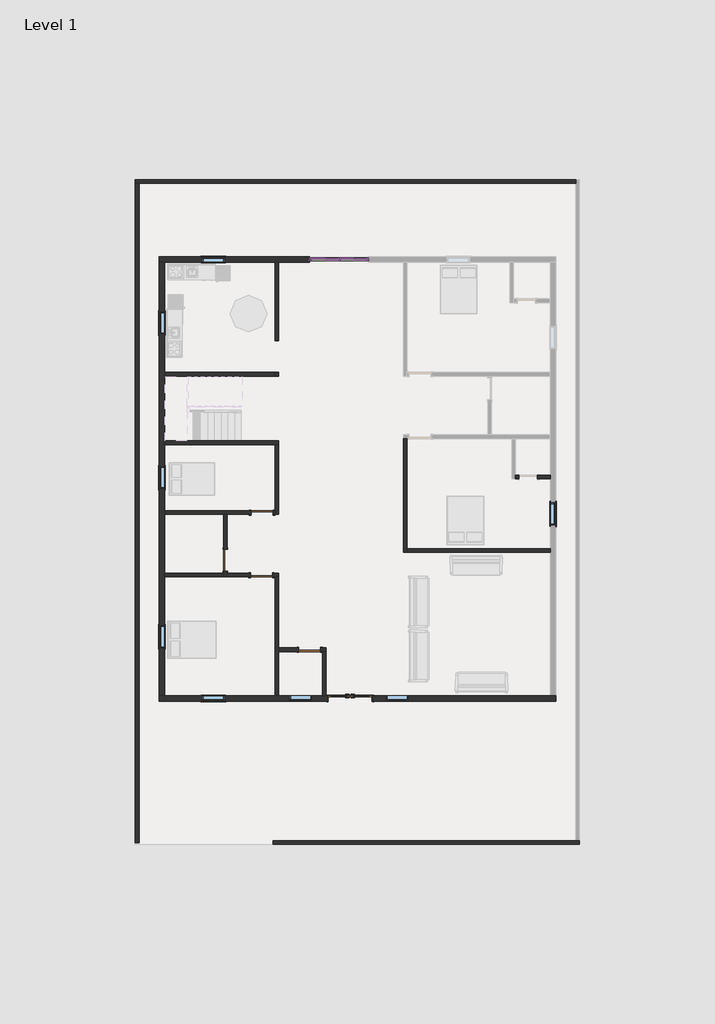
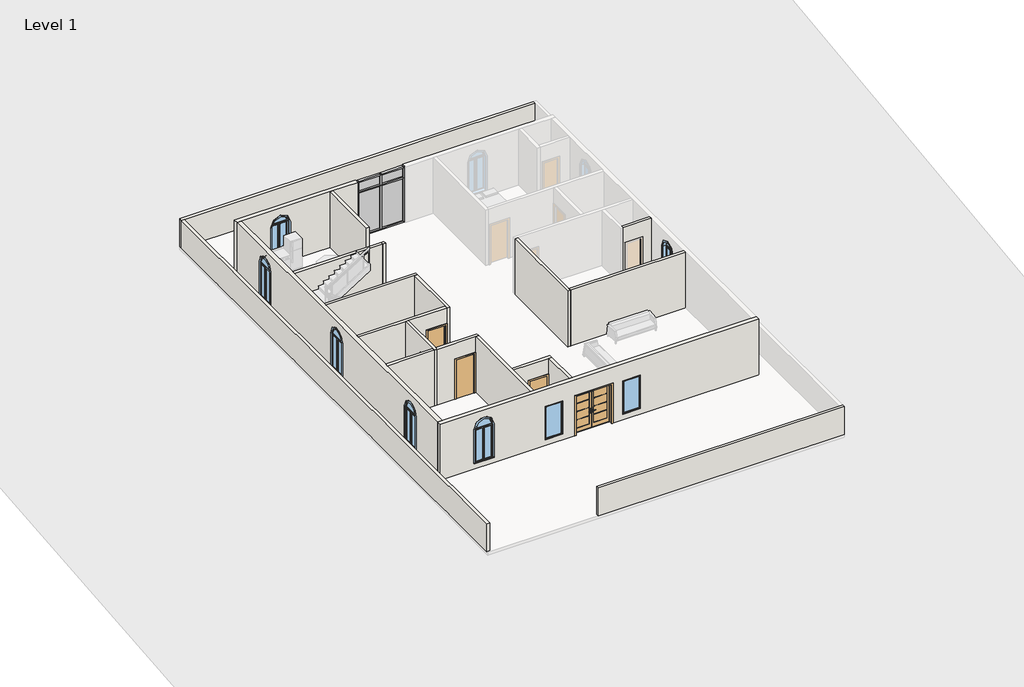
# One storey, part 1 of 2: 21 walls, 12 members, 8 windows, 5 doors, 4 plates.
"""IFC4 building model written with IfcOpenShell, lengths in millimetres."""

from ifc_helpers import new_model, si_unit, frame, origin, origin_with_axes, place, context, project, spatial, polyline, circle_curve, outline, extrude, faceted_brep, transform, mapped, element, save
from ifc_brep_helpers import plane_surface, revolved_surface, advanced_brep
from components import door_5bfea099, door_686f89d2, door_16372e1c, member_e6b9f524, member_866a01fa, member_f0fea5a5, member_6e77e263, member_ee409385, member_47bfaf8a, system_panel_glazed_2148303e, system_panel_glazed_80d043f3, window_e7489165, window_c796fc87

model = new_model("IFC4")

# Units and contexts
model_context = context("Model", 3, world=origin())
ifc_project = project(units=[si_unit("LENGTHUNIT", "METRE", prefix="MILLI")], contexts=[model_context])

# Site, building, storey
site = spatial("IfcSite", under=ifc_project)
building = spatial("IfcBuilding", under=site)
storey = spatial("IfcBuildingStorey", under=building, Name="Level 1", Elevation=0.0)

# Doors
placement = place(None, origin())
door_shape = door_5bfea099(model_context)
element("IfcDoor", 1, ObjectType="Door-Exterior-Double-Full Glass-Wood_Clad : 72\" x 84\"", at=placement, inside=storey, context=model_context, shape_type="MappedRepresentation", body=[
    mapped(door_shape, transform((-1367.6791271, -5663.3296952, 0.0), x_axis=(1.0, 0.0, 0.0), y_axis=(0.0, 1.0, 0.0), z_axis=(0.0, 0.0, 1.0))),
])
door_2_shape = door_686f89d2(model_context)
element("IfcDoor", 2, ObjectType="Single-Flush : 36\" x 84\"", at=placement, inside=storey, context=model_context, shape_type="MappedRepresentation", body=[
    mapped(door_2_shape, transform((-5050.6791271, -548.4046952, 0.0), x_axis=(1.0, 0.0, 0.0), y_axis=(0.0, 1.0, 0.0), z_axis=(0.0, 0.0, 1.0))),
])
element("IfcDoor", 3, ObjectType="Single-Flush : 36\" x 84\"", at=placement, inside=storey, context=model_context, shape_type="MappedRepresentation", body=[
    mapped(door_2_shape, transform((-6549.2791271, 61.1953048, 0.0), x_axis=(0.0, -1.0, 0.0), y_axis=(1.0, 0.0, 0.0), z_axis=(0.0, 0.0, 1.0))),
])
element("IfcDoor", 4, ObjectType="Single-Flush : 36\" x 84\"", at=placement, inside=storey, context=model_context, shape_type="MappedRepresentation", body=[
    mapped(door_2_shape, transform((-3044.0791271, -3647.2046952, 0.0), x_axis=(1.0, 0.0, 0.0), y_axis=(0.0, 1.0, 0.0), z_axis=(0.0, 0.0, 1.0))),
])
door_3_shape = door_16372e1c(model_context)
element("IfcDoor", 5, ObjectType="Single-Flush : 36\" x 84\"", at=placement, inside=storey, context=model_context, shape_type="MappedRepresentation", body=[
    mapped(door_3_shape, transform((-5025.2791271, 2042.3953048, 0.0), x_axis=(1.0, 0.0, 0.0), y_axis=(0.0, 1.0, 0.0), z_axis=(0.0, 0.0, 1.0))),
])

# Members
member_shape = member_e6b9f524(model_context)
element("IfcMember", 6, ObjectType="Rectangular Mullion : 2.5\" x 5\" rectangular", at=placement, inside=storey, context=model_context, shape_type="MappedRepresentation", body=[
    mapped(member_shape, transform((-669.1791271, 12545.2953048, 3048.0), x_axis=(0.0, 0.0, 1.0), y_axis=(0.0, -1.0, 0.0), z_axis=(1.0, 0.0, 0.0))),
])
element("IfcMember", 7, ObjectType="Rectangular Mullion : 2.5\" x 5\" rectangular", at=placement, inside=storey, context=model_context, shape_type="MappedRepresentation", body=[
    mapped(member_shape, transform((-1856.6291271, 12545.2953048, 3048.0), x_axis=(0.0, 0.0, 1.0), y_axis=(0.0, -1.0, 0.0), z_axis=(1.0, 0.0, 0.0))),
])
element("IfcMember", 8, ObjectType="Rectangular Mullion : 2.5\" x 5\" rectangular", at=placement, inside=storey, context=model_context, shape_type="MappedRepresentation", body=[
    mapped(member_shape, transform((-2980.5791271, 12545.2953048, 0.0), x_axis=(0.0, 0.0, -1.0), y_axis=(0.0, -1.0, 0.0), z_axis=(-1.0, 0.0, 0.0))),
])
element("IfcMember", 9, ObjectType="Rectangular Mullion : 2.5\" x 5\" rectangular", at=placement, inside=storey, context=model_context, shape_type="MappedRepresentation", body=[
    mapped(member_shape, transform((-1793.1291271, 12545.2953048, 0.0), x_axis=(0.0, 0.0, -1.0), y_axis=(0.0, -1.0, 0.0), z_axis=(-1.0, 0.0, 0.0))),
])
member_2_shape = member_866a01fa(model_context)
element("IfcMember", 10, ObjectType="Rectangular Mullion : 2.5\" x 5\" rectangular", at=placement, inside=storey, context=model_context, shape_type="MappedRepresentation", body=[
    mapped(member_2_shape, transform((-1856.6291271, 12545.2953048, 2438.4), x_axis=(0.0, 0.0, 1.0), y_axis=(0.0, -1.0, 0.0), z_axis=(1.0, 0.0, 0.0))),
])
element("IfcMember", 11, ObjectType="Rectangular Mullion : 2.5\" x 5\" rectangular", at=placement, inside=storey, context=model_context, shape_type="MappedRepresentation", body=[
    mapped(member_2_shape, transform((-669.1791271, 12545.2953048, 2438.4), x_axis=(0.0, 0.0, 1.0), y_axis=(0.0, -1.0, 0.0), z_axis=(1.0, 0.0, 0.0))),
])
member_3_shape = member_f0fea5a5(model_context)
element("IfcMember", 12, ObjectType="Rectangular Mullion : 2.5\" x 5\" rectangular", at=placement, inside=storey, context=model_context, shape_type="MappedRepresentation", body=[
    mapped(member_3_shape, transform((-1824.8791271, 12545.2953048, 0.0), x_axis=(1.0, 0.0, 0.0), y_axis=(0.0, -1.0, 0.0), z_axis=(0.0, 0.0, -1.0))),
])
member_4_shape = member_6e77e263(model_context)
element("IfcMember", 13, ObjectType="Rectangular Mullion : 2.5\" x 5\" rectangular", at=placement, inside=storey, context=model_context, shape_type="MappedRepresentation", body=[
    mapped(member_4_shape, transform((-1824.8791271, 12545.2953048, 2438.4), x_axis=(1.0, 0.0, 0.0), y_axis=(0.0, -1.0, 0.0), z_axis=(0.0, 0.0, -1.0))),
])
member_5_shape = member_ee409385(model_context)
element("IfcMember", 14, ObjectType="Rectangular Mullion : 2.5\" x 5\" rectangular", at=placement, inside=storey, context=model_context, shape_type="MappedRepresentation", body=[
    mapped(member_5_shape, transform((-605.6791271, 12545.2953048, 0.0), x_axis=(1.0, 0.0, 0.0), y_axis=(0.0, -1.0, 0.0), z_axis=(0.0, 0.0, -1.0))),
])
member_6_shape = member_47bfaf8a(model_context)
element("IfcMember", 15, ObjectType="Rectangular Mullion : 2.5\" x 5\" rectangular", at=placement, inside=storey, context=model_context, shape_type="MappedRepresentation", body=[
    mapped(member_6_shape, transform((-3044.0791271, 12545.2953048, 3048.0), x_axis=(-1.0, 0.0, 0.0), y_axis=(0.0, -1.0, 0.0), z_axis=(0.0, 0.0, 1.0))),
])
element("IfcMember", 16, ObjectType="Rectangular Mullion : 2.5\" x 5\" rectangular", at=placement, inside=storey, context=model_context, shape_type="MappedRepresentation", body=[
    mapped(member_6_shape, transform((-605.6791271, 12545.2953048, 2438.4), x_axis=(1.0, 0.0, 0.0), y_axis=(0.0, -1.0, 0.0), z_axis=(0.0, 0.0, -1.0))),
])
element("IfcMember", 17, ObjectType="Rectangular Mullion : 2.5\" x 5\" rectangular", at=placement, inside=storey, context=model_context, shape_type="MappedRepresentation", body=[
    mapped(member_5_shape, transform((-3044.0791271, 12545.2953048, 2438.4), x_axis=(-1.0, 0.0, 0.0), y_axis=(0.0, -1.0, 0.0), z_axis=(0.0, 0.0, 1.0))),
])

# Plates
system_panel_glazed_shape = system_panel_glazed_2148303e(model_context)
element("IfcPlate", 18, ObjectType="System Panel : Glazed", at=placement, inside=storey, context=model_context, shape_type="MappedRepresentation", body=[
    mapped(system_panel_glazed_shape, transform((-2418.6041271, 12545.2953048, 63.5), x_axis=(1.0, 0.0, 0.0), y_axis=(0.0, 1.0, 0.0), z_axis=(0.0, 0.0, 1.0))),
])
element("IfcPlate", 19, ObjectType="System Panel : Glazed", at=placement, inside=storey, context=model_context, shape_type="MappedRepresentation", body=[
    mapped(system_panel_glazed_shape, transform((-1231.1541271, 12545.2953048, 63.5), x_axis=(1.0, 0.0, 0.0), y_axis=(0.0, 1.0, 0.0), z_axis=(0.0, 0.0, 1.0))),
])
system_panel_glazed_2_shape = system_panel_glazed_80d043f3(model_context)
element("IfcPlate", 20, ObjectType="System Panel : Glazed", at=placement, inside=storey, context=model_context, shape_type="MappedRepresentation", body=[
    mapped(system_panel_glazed_2_shape, transform((-2418.6041271, 12545.2953048, 2470.15), x_axis=(1.0, 0.0, 0.0), y_axis=(0.0, 1.0, 0.0), z_axis=(0.0, 0.0, 1.0))),
])
element("IfcPlate", 21, ObjectType="System Panel : Glazed", at=placement, inside=storey, context=model_context, shape_type="MappedRepresentation", body=[
    mapped(system_panel_glazed_2_shape, transform((-1231.1541271, 12545.2953048, 2470.15), x_axis=(1.0, 0.0, 0.0), y_axis=(0.0, 1.0, 0.0), z_axis=(0.0, 0.0, 1.0))),
])

# Walls
element("IfcWall", 22, ObjectType="6\"", at=placement, inside=storey, context=model_context, shape_type="Brep", body=[
    faceted_brep([(-10283.0791271, 15707.5953048, 0.0), (-10130.6791271, 15707.5953048, 0.0), (8004.9208729, 15707.5953048, 0.0), (8004.9208729, 15707.5953048, 1524.0), (-10130.6791271, 15707.5953048, 1524.0), (-10283.0791271, 15707.5953048, 1524.0), (-10283.0791271, 15859.9953048, 0.0), (-10283.0791271, 15859.9953048, 1524.0), (8004.9208729, 15859.9953048, 1524.0), (8004.9208729, 15859.9953048, 0.0)], [[[0, 1, 2, 3, 4, 5]], [[6, 7, 8, 9]], [[2, 1, 0, 6, 9]], [[5, 4, 3, 8, 7]], [[0, 5, 7, 6]], [[3, 2, 9, 8]]]),
])
element("IfcWall", 23, ObjectType="6\"", at=placement, inside=storey, context=model_context, shape_type="SweptSolid", body=[
    extrude(outline(polyline([(-10130.6791271, 15707.5953048), (-10130.6791271, -11648.2046952), (-10283.0791271, -11648.2046952), (-10283.0791271, 15707.5953048), (-10130.6791271, 15707.5953048)])), origin_with_axes(), (0.0, 0.0, 1.0), 1524.0),
])
element("IfcWall", 24, ObjectType="6\"", at=placement, inside=storey, context=model_context, shape_type="Brep", body=[
    faceted_brep([(8157.3208729, -11572.0046952, 0.0), (8004.9208729, -11572.0046952, 0.0), (-4568.0791271, -11572.0046952, 0.0), (-4568.0791271, -11572.0046952, 1524.0), (8004.9208729, -11572.0046952, 1524.0), (8157.3208729, -11572.0046952, 1524.0), (8157.3208729, -11724.4046952, 0.0), (8157.3208729, -11724.4046952, 1524.0), (-4568.0791271, -11724.4046952, 1524.0), (-4568.0791271, -11724.4046952, 0.0)], [[[0, 1, 2, 3, 4, 5]], [[6, 7, 8, 9]], [[2, 1, 0, 6, 9]], [[3, 2, 9, 8]], [[5, 4, 3, 8, 7]], [[0, 5, 7, 6]]]),
])
element("IfcWall", 25, ObjectType="6\"", at=placement, inside=storey, context=model_context, shape_type="SweptSolid", body=[
    extrude(outline(polyline([(-4491.8791271, 9167.0953048), (-4491.8791271, 12430.9953048), (-4339.4791271, 12430.9953048), (-4339.4791271, 9167.0953048), (-4491.8791271, 9167.0953048)])), origin_with_axes(), (0.0, 0.0, 1.0), 3048.0),
])
element("IfcWall", 26, ObjectType="6\"", at=placement, inside=storey, context=model_context, shape_type="SweptSolid", body=[
    extrude(outline(polyline([(-9063.8791271, 7858.9953048), (-4491.8791271, 7858.9953048), (-4491.8791271, 7706.5953048), (-9063.8791271, 7706.5953048), (-9063.8791271, 7858.9953048)])), origin_with_axes(), (0.0, 0.0, 1.0), 3048.0),
])
element("IfcWall", 27, ObjectType="6\"", at=placement, inside=storey, context=model_context, shape_type="Brep", body=[
    faceted_brep([(842.1208729, 5115.7953048, 0.0), (842.1208729, 391.3953048, 0.0), (842.1208729, 391.3953048, 3048.0), (842.1208729, 5115.7953048, 3048.0), (994.5208729, 5115.7953048, 0.0), (994.5208729, 5115.7953048, 3048.0), (994.5208729, 543.7953048, 3048.0), (994.5208729, 391.3953048, 3048.0), (994.5208729, 391.3953048, 0.0), (994.5208729, 543.7953048, 0.0)], [[[0, 1, 2, 3]], [[4, 5, 6, 7, 8, 9]], [[1, 0, 4, 9, 8]], [[3, 2, 7, 6, 5]], [[2, 1, 8, 7]], [[0, 3, 5, 4]]]),
])
element("IfcWall", 28, ObjectType="6\"", at=placement, inside=storey, context=model_context, shape_type="SweptSolid", body=[
    extrude(outline(polyline([(6938.1208729, 391.3953048), (994.5208729, 391.3953048), (994.5208729, 543.7953048), (6938.1208729, 543.7953048), (6938.1208729, 391.3953048)])), origin_with_axes(), (0.0, 0.0, 1.0), 3048.0),
])
element("IfcWall", 29, ObjectType="6\"", at=placement, inside=storey, context=model_context, shape_type="Brep", body=[
    faceted_brep([(-9063.8791271, 4861.7953048, 0.0), (-4491.8791271, 4861.7953048, 0.0), (-4339.4791271, 4861.7953048, 0.0), (-4339.4791271, 4861.7953048, 3048.0), (-4491.8791271, 4861.7953048, 3048.0), (-9063.8791271, 4861.7953048, 3048.0), (-9063.8791271, 5014.1953048, 0.0), (-9063.8791271, 5014.1953048, 3048.0), (-4339.4791271, 5014.1953048, 3048.0), (-4339.4791271, 5014.1953048, 0.0)], [[[0, 1, 2, 3, 4, 5]], [[6, 7, 8, 9]], [[2, 1, 0, 6, 9]], [[5, 4, 3, 8, 7]], [[3, 2, 9, 8]], [[0, 5, 7, 6]]]),
])
element("IfcWall", 30, ObjectType="6\"", at=placement, inside=storey, context=model_context, shape_type="Brep", body=[
    faceted_brep([(-4491.8791271, 4861.7953048, 0.0), (-4491.8791271, 2118.5953048, 0.0), (-4491.8791271, 1966.1953048, 0.0), (-4491.8791271, 1966.1953048, 3048.0), (-4491.8791271, 2118.5953048, 3048.0), (-4491.8791271, 4861.7953048, 3048.0), (-4339.4791271, 4861.7953048, 0.0), (-4339.4791271, 4861.7953048, 3048.0), (-4339.4791271, 1966.1953048, 3048.0), (-4339.4791271, 1966.1953048, 0.0)], [[[0, 1, 2, 3, 4, 5]], [[6, 7, 8, 9]], [[2, 1, 0, 6, 9]], [[5, 4, 3, 8, 7]], [[0, 5, 7, 6]], [[3, 2, 9, 8]]]),
])
element("IfcWall", 31, ObjectType="6\"", at=placement, inside=storey, context=model_context, shape_type="Brep", body=[
    faceted_brep([(-4491.8791271, 2118.5953048, 0.0), (-4568.0791271, 2118.5953048, 0.0), (-4568.0791271, 2118.5953048, 2133.6), (-5482.4791271, 2118.5953048, 2133.6), (-5482.4791271, 2118.5953048, 0.0), (-9063.8791271, 2118.5953048, 0.0), (-9063.8791271, 2118.5953048, 3048.0), (-4491.8791271, 2118.5953048, 3048.0), (-4568.0791271, 1966.1953048, 2133.6), (-4568.0791271, 1966.1953048, 0.0), (-4491.8791271, 1966.1953048, 0.0), (-4491.8791271, 1966.1953048, 3048.0), (-6473.0791271, 1966.1953048, 3048.0), (-6625.4791271, 1966.1953048, 3048.0), (-9063.8791271, 1966.1953048, 3048.0), (-9063.8791271, 1966.1953048, 0.0), (-6625.4791271, 1966.1953048, 0.0), (-6473.0791271, 1966.1953048, 0.0), (-5482.4791271, 1966.1953048, 0.0), (-5482.4791271, 1966.1953048, 2133.6)], [[[0, 1, 2, 3, 4, 5, 6, 7]], [[8, 9, 10, 11, 12, 13, 14, 15, 16, 17, 18, 19]], [[10, 9, 1, 0]], [[18, 17, 16, 15, 5, 4]], [[7, 6, 14, 13, 12, 11]], [[0, 7, 11, 10]], [[6, 5, 15, 14]], [[2, 1, 9, 8]], [[3, 2, 8, 19]], [[4, 3, 19, 18]]]),
])
element("IfcWall", 32, ObjectType="6\"", at=placement, inside=storey, context=model_context, shape_type="Brep", body=[
    faceted_brep([(-6625.4791271, -396.0046952, 2133.6), (-6625.4791271, -396.0046952, 0.0), (-6625.4791271, -472.2046952, 0.0), (-6625.4791271, -624.6046952, 0.0), (-6625.4791271, -624.6046952, 3048.0), (-6625.4791271, -472.2046952, 3048.0), (-6625.4791271, 1966.1953048, 3048.0), (-6625.4791271, 1966.1953048, 0.0), (-6625.4791271, 518.3953048, 0.0), (-6625.4791271, 518.3953048, 2133.6), (-6473.0791271, -624.6046952, 0.0), (-6473.0791271, -472.2046952, 0.0), (-6473.0791271, -396.0046952, 0.0), (-6473.0791271, -396.0046952, 2133.6), (-6473.0791271, 518.3953048, 2133.6), (-6473.0791271, 518.3953048, 0.0), (-6473.0791271, 1966.1953048, 0.0), (-6473.0791271, 1966.1953048, 3048.0), (-6473.0791271, -472.2046952, 3048.0), (-6473.0791271, -624.6046952, 3048.0)], [[[0, 1, 2, 3, 4, 5, 6, 7, 8, 9]], [[10, 11, 12, 13, 14, 15, 16, 17, 18, 19]], [[8, 7, 16, 15]], [[3, 2, 1, 12, 11, 10]], [[6, 5, 4, 19, 18, 17]], [[7, 6, 17, 16]], [[4, 3, 10, 19]], [[13, 12, 1, 0]], [[14, 13, 0, 9]], [[15, 14, 9, 8]]]),
])
element("IfcWall", 33, ObjectType="6\"", at=placement, inside=storey, context=model_context, shape_type="SweptSolid", body=[
    extrude(outline(polyline([(-9063.8791271, -472.2046952), (-6625.4791271, -472.2046952), (-6625.4791271, -624.6046952), (-9063.8791271, -624.6046952), (-9063.8791271, -472.2046952)])), origin_with_axes(), (0.0, 0.0, 1.0), 3048.0),
])
element("IfcWall", 34, ObjectType="6\"", at=placement, inside=storey, context=model_context, shape_type="Brep", body=[
    faceted_brep([(-4593.4791271, -624.6046952, 2133.6), (-4593.4791271, -624.6046952, 0.0), (-4491.8791271, -624.6046952, 0.0), (-4339.4791271, -624.6046952, 0.0), (-4339.4791271, -624.6046952, 3048.0), (-4491.8791271, -624.6046952, 3048.0), (-6473.0791271, -624.6046952, 3048.0), (-6473.0791271, -624.6046952, 0.0), (-5507.8791271, -624.6046952, 0.0), (-5507.8791271, -624.6046952, 2133.6), (-4339.4791271, -472.2046952, 0.0), (-4593.4791271, -472.2046952, 0.0), (-4593.4791271, -472.2046952, 2133.6), (-5507.8791271, -472.2046952, 2133.6), (-5507.8791271, -472.2046952, 0.0), (-6473.0791271, -472.2046952, 0.0), (-6473.0791271, -472.2046952, 3048.0), (-4339.4791271, -472.2046952, 3048.0)], [[[0, 1, 2, 3, 4, 5, 6, 7, 8, 9]], [[10, 11, 12, 13, 14, 15, 16, 17]], [[8, 7, 15, 14]], [[3, 2, 1, 11, 10]], [[6, 5, 4, 17, 16]], [[7, 6, 16, 15]], [[4, 3, 10, 17]], [[12, 11, 1, 0]], [[13, 12, 0, 9]], [[14, 13, 9, 8]]]),
])
element("IfcWall", 35, ObjectType="6\"", at=placement, inside=storey, context=model_context, shape_type="Brep", body=[
    faceted_brep([(-4491.8791271, -624.6046952, 0.0), (-4491.8791271, -5552.2046952, 0.0), (-4491.8791271, -5552.2046952, 3048.0), (-4491.8791271, -624.6046952, 3048.0), (-4339.4791271, -624.6046952, 0.0), (-4339.4791271, -624.6046952, 3048.0), (-4339.4791271, -3571.0046952, 3048.0), (-4339.4791271, -3723.4046952, 3048.0), (-4339.4791271, -5552.2046952, 3048.0), (-4339.4791271, -5552.2046952, 0.0), (-4339.4791271, -3723.4046952, 0.0), (-4339.4791271, -3571.0046952, 0.0)], [[[0, 1, 2, 3]], [[4, 5, 6, 7, 8, 9, 10, 11]], [[1, 0, 4, 11, 10, 9]], [[3, 2, 8, 7, 6, 5]], [[0, 3, 5, 4]], [[2, 1, 9, 8]]]),
])
element("IfcWall", 36, ObjectType="6\"", at=placement, inside=storey, context=model_context, shape_type="Brep", body=[
    faceted_brep([(-2586.8791271, -3723.4046952, 2133.6), (-2586.8791271, -3723.4046952, 0.0), (-2510.6791271, -3723.4046952, 0.0), (-2358.2791271, -3723.4046952, 0.0), (-2358.2791271, -3723.4046952, 3048.0), (-2510.6791271, -3723.4046952, 3048.0), (-4339.4791271, -3723.4046952, 3048.0), (-4339.4791271, -3723.4046952, 0.0), (-3501.2791271, -3723.4046952, 0.0), (-3501.2791271, -3723.4046952, 2133.6), (-2358.2791271, -3571.0046952, 0.0), (-2586.8791271, -3571.0046952, 0.0), (-2586.8791271, -3571.0046952, 2133.6), (-3501.2791271, -3571.0046952, 2133.6), (-3501.2791271, -3571.0046952, 0.0), (-4339.4791271, -3571.0046952, 0.0), (-4339.4791271, -3571.0046952, 3048.0), (-2358.2791271, -3571.0046952, 3048.0)], [[[0, 1, 2, 3, 4, 5, 6, 7, 8, 9]], [[10, 11, 12, 13, 14, 15, 16, 17]], [[8, 7, 15, 14]], [[3, 2, 1, 11, 10]], [[6, 5, 4, 17, 16]], [[7, 6, 16, 15]], [[4, 3, 10, 17]], [[12, 11, 1, 0]], [[13, 12, 0, 9]], [[14, 13, 9, 8]]]),
])
element("IfcWall", 37, ObjectType="6\"", at=placement, inside=storey, context=model_context, shape_type="SweptSolid", body=[
    extrude(outline(polyline([(-2510.6791271, -5552.2046952), (-2510.6791271, -3723.4046952), (-2358.2791271, -3723.4046952), (-2358.2791271, -5552.2046952), (-2510.6791271, -5552.2046952)])), origin_with_axes(), (0.0, 0.0, 1.0), 3048.0),
])
element("IfcWall", 38, ObjectType="6\"", at=placement, inside=storey, context=model_context, shape_type="SweptSolid", body=[
    extrude(outline(polyline([(0.0, 5490.3208729), (0.0, 5642.7208729), (2133.6, 5642.7208729), (2133.6, 6404.7208729), (0.0, 6404.7208729), (0.0, 6938.1208729), (3048.0, 6938.1208729), (3048.0, 5490.3208729), (0.0, 5490.3208729)])), frame((0.0, 3439.3953048, 0.0), z_axis=(0.0, 1.0, 0.0), x_axis=(0.0, 0.0, 1.0)), (0.0, 0.0, 1.0), 152.4),
])
element("IfcWall", 39, ObjectType="6\"", at=placement, inside=storey, context=model_context, shape_type="SweptSolid", body=[
    extrude(outline(polyline([(-4491.8791271, 7706.5953048), (-4491.8791271, 7858.9953048), (-4339.4791271, 7858.9953048), (-4339.4791271, 7706.5953048), (-4491.8791271, 7706.5953048)])), origin_with_axes(), (0.0, 0.0, 1.0), 3048.0),
])
element("IfcWall", 40, ObjectType="9\"", at=placement, inside=storey, context=model_context, shape_type="AdvancedBrep", body=[
    advanced_brep(
    [(-9292.4791271, 12430.9953048, 0.0), (-9063.8791271, 12430.9953048, 0.0), (-4491.8791271, 12430.9953048, 0.0), (-4339.4791271, 12430.9953048, 0.0), (-3044.0791271, 12430.9953048, 0.0), (-3044.0791271, 12430.9953048, 3048.0), (-4339.4791271, 12430.9953048, 3048.0), (-4491.8791271, 12430.9953048, 3048.0), (-9063.8791271, 12430.9953048, 3048.0), (-9292.4791271, 12430.9953048, 3048.0), (-6587.3791271, 12430.9953048, 2152.65), (-6587.3791271, 12430.9953048, 304.8), (-7501.7791271, 12430.9953048, 304.8), (-7501.7791271, 12430.9953048, 2152.65), (-9292.4791271, 12659.5953048, 0.0), (-9292.4791271, 12659.5953048, 3048.0), (-3044.0791271, 12659.5953048, 3048.0), (-3044.0791271, 12659.5953048, 0.0), (-6587.3791271, 12659.5953048, 2152.65), (-7501.7791271, 12659.5953048, 2152.65), (-7501.7791271, 12659.5953048, 304.8), (-6587.3791271, 12659.5953048, 304.8)],
    [
        (0, 1),
        (1, 2),
        (2, 3),
        (3, 4),
        (4, 5),
        (5, 6),
        (6, 7),
        (7, 8),
        (8, 9),
        (9, 0),
        (10, 11),
        (11, 12),
        (12, 13),
        (13, 10, circle_curve(frame((-7044.5791271, 12430.9953048, 2152.65), z_axis=(0.0, 1.0, 0.0), x_axis=(1.0, 0.0, 0.0)), 457.2)),
        (14, 15),
        (15, 16),
        (16, 17),
        (17, 14),
        (18, 19, circle_curve(frame((-7044.5791271, 12659.5953048, 2152.65), z_axis=(0.0, -1.0, 0.0), x_axis=(1.0, 0.0, 0.0)), 457.2)),
        (19, 20),
        (20, 21),
        (21, 18),
        (0, 14),
        (17, 4),
        (16, 5),
        (15, 9),
        (10, 18),
        (21, 11),
        (20, 12),
        (19, 13),
    ],
    [
        plane_surface(frame((-10130.6791271, 12430.9953048, 0.0), z_axis=(0.0, -1.0, 0.0), x_axis=(1.0, 0.0, 0.0))),
        plane_surface(frame((-10130.6791271, 12659.5953048, 0.0), z_axis=(0.0, 1.0, 0.0), x_axis=(-1.0, 0.0, 0.0))),
        plane_surface(frame((-9292.4791271, 12430.9953048, 0.0), z_axis=(0.0, 0.0, -1.0), x_axis=(0.0, 1.0, 0.0))),
        plane_surface(frame((-3044.0791271, 12430.9953048, 0.0), z_axis=(1.0, 0.0, 0.0), x_axis=(0.0, 1.0, 0.0))),
        plane_surface(frame((-3044.0791271, 12430.9953048, 3048.0), z_axis=(0.0, 0.0, 1.0), x_axis=(0.0, 1.0, 0.0))),
        plane_surface(frame((-9292.4791271, 12430.9953048, 3048.0), z_axis=(-1.0, 0.0, 0.0), x_axis=(0.0, 1.0, 0.0))),
        plane_surface(frame((-6587.3791271, 12430.9953048, 2152.65), z_axis=(-1.0, 0.0, 0.0), x_axis=(0.0, 1.0, 0.0))),
        plane_surface(frame((-6587.3791271, 12430.9953048, 304.8), z_axis=(0.0, 0.0, 1.0), x_axis=(0.0, 1.0, 0.0))),
        plane_surface(frame((-7501.7791271, 12430.9953048, 304.8), z_axis=(1.0, 0.0, 0.0), x_axis=(0.0, 1.0, 0.0))),
        revolved_surface(polyline([(-6587.3791271, 12659.5953048, 2152.65), (-6587.3791271, 12430.9953048, 2152.65)]), (-7044.5791271, 12430.9953048, 2152.65), (0.0, 1.0, 0.0)),
    ],
    [
        (0, [[1, 2, 3, 4, 5, 6, 7, 8, 9, 10], [11, 12, 13, 14]]),
        (1, [[15, 16, 17, 18], [19, 20, 21, 22]]),
        (2, [[-4, -3, -2, -1, 23, -18, 24]]),
        (3, [[-5, -24, -17, 25]]),
        (4, [[-9, -8, -7, -6, -25, -16, 26]]),
        (5, [[-10, -26, -15, -23]]),
        (6, [[-11, 27, -22, 28]]),
        (7, [[-12, -28, -21, 29]]),
        (8, [[-13, -29, -20, 30]]),
        (9, [[-14, -30, -19, -27]]),
    ],
),
])
element("IfcWall", 41, ObjectType="9\"", at=placement, inside=storey, context=model_context, shape_type="AdvancedBrep", body=[
    advanced_brep(
    [(-9292.4791271, 12430.9953048, 0.0), (-9292.4791271, -5552.2046952, 0.0), (-9292.4791271, -5552.2046952, 3048.0), (-9292.4791271, 12430.9953048, 3048.0), (-9292.4791271, -2650.2546952, 2152.65), (-9292.4791271, -3564.6546952, 2152.65), (-9292.4791271, -3564.6546952, 304.8), (-9292.4791271, -2650.2546952, 304.8), (-9292.4791271, 3947.3953048, 2152.65), (-9292.4791271, 3032.9953048, 2152.65), (-9292.4791271, 3032.9953048, 304.8), (-9292.4791271, 3947.3953048, 304.8), (-9292.4791271, 10367.2453048, 2152.65), (-9292.4791271, 9452.8453048, 2152.65), (-9292.4791271, 9452.8453048, 304.8), (-9292.4791271, 10367.2453048, 304.8), (-9063.8791271, 12430.9953048, 0.0), (-9063.8791271, 12430.9953048, 3048.0), (-9063.8791271, 7858.9953048, 3048.0), (-9063.8791271, 7706.5953048, 3048.0), (-9063.8791271, 5014.1953048, 3048.0), (-9063.8791271, 4861.7953048, 3048.0), (-9063.8791271, 2118.5953048, 3048.0), (-9063.8791271, 1966.1953048, 3048.0), (-9063.8791271, -472.2046952, 3048.0), (-9063.8791271, -624.6046952, 3048.0), (-9063.8791271, -5552.2046952, 3048.0), (-9063.8791271, -5552.2046952, 0.0), (-9063.8791271, -624.6046952, 0.0), (-9063.8791271, -472.2046952, 0.0), (-9063.8791271, 1966.1953048, 0.0), (-9063.8791271, 2118.5953048, 0.0), (-9063.8791271, 4861.7953048, 0.0), (-9063.8791271, 5014.1953048, 0.0), (-9063.8791271, 7706.5953048, 0.0), (-9063.8791271, 7858.9953048, 0.0), (-9063.8791271, -2650.2546952, 2152.65), (-9063.8791271, -2650.2546952, 304.8), (-9063.8791271, -3564.6546952, 304.8), (-9063.8791271, -3564.6546952, 2152.65), (-9063.8791271, 3947.3953048, 2152.65), (-9063.8791271, 3947.3953048, 304.8), (-9063.8791271, 3032.9953048, 304.8), (-9063.8791271, 3032.9953048, 2152.65), (-9063.8791271, 10367.2453048, 2152.65), (-9063.8791271, 10367.2453048, 304.8), (-9063.8791271, 9452.8453048, 304.8), (-9063.8791271, 9452.8453048, 2152.65)],
    [
        (0, 1),
        (1, 2),
        (2, 3),
        (3, 0),
        (4, 5, circle_curve(frame((-9292.4791271, -3107.4546952, 2152.65), z_axis=(1.0, 0.0, 0.0), x_axis=(0.0, 1.0, 0.0)), 457.2)),
        (5, 6),
        (6, 7),
        (7, 4),
        (8, 9, circle_curve(frame((-9292.4791271, 3490.1953048, 2152.65), z_axis=(1.0, 0.0, 0.0), x_axis=(0.0, 1.0, 0.0)), 457.2)),
        (9, 10),
        (10, 11),
        (11, 8),
        (12, 13, circle_curve(frame((-9292.4791271, 9910.0453048, 2152.65), z_axis=(1.0, 0.0, 0.0), x_axis=(0.0, 1.0, 0.0)), 457.2)),
        (13, 14),
        (14, 15),
        (15, 12),
        (16, 17),
        (17, 18),
        (18, 19),
        (19, 20),
        (20, 21),
        (21, 22),
        (22, 23),
        (23, 24),
        (24, 25),
        (25, 26),
        (26, 27),
        (27, 28),
        (28, 29),
        (29, 30),
        (30, 31),
        (31, 32),
        (32, 33),
        (33, 34),
        (34, 35),
        (35, 16),
        (36, 37),
        (37, 38),
        (38, 39),
        (39, 36, circle_curve(frame((-9063.8791271, -3107.4546952, 2152.65), z_axis=(-1.0, 0.0, 0.0), x_axis=(0.0, 1.0, 0.0)), 457.2)),
        (40, 41),
        (41, 42),
        (42, 43),
        (43, 40, circle_curve(frame((-9063.8791271, 3490.1953048, 2152.65), z_axis=(-1.0, 0.0, 0.0), x_axis=(0.0, 1.0, 0.0)), 457.2)),
        (44, 45),
        (45, 46),
        (46, 47),
        (47, 44, circle_curve(frame((-9063.8791271, 9910.0453048, 2152.65), z_axis=(-1.0, 0.0, 0.0), x_axis=(0.0, 1.0, 0.0)), 457.2)),
        (0, 16),
        (27, 1),
        (2, 26),
        (17, 3),
        (36, 4),
        (7, 37),
        (6, 38),
        (5, 39),
        (40, 8),
        (11, 41),
        (10, 42),
        (9, 43),
        (44, 12),
        (15, 45),
        (14, 46),
        (13, 47),
    ],
    [
        plane_surface(frame((-9292.4791271, 12430.9953048, 0.0), z_axis=(-1.0, 0.0, 0.0), x_axis=(0.0, -1.0, 0.0))),
        plane_surface(frame((-9063.8791271, 12430.9953048, 0.0), z_axis=(1.0, 0.0, 0.0), x_axis=(0.0, 1.0, 0.0))),
        plane_surface(frame((-9292.4791271, 12545.2953048, 0.0), z_axis=(0.0, 0.0, -1.0), x_axis=(1.0, 0.0, 0.0))),
        plane_surface(frame((-9292.4791271, -5666.5046952, 3048.0), z_axis=(0.0, 0.0, 1.0), x_axis=(1.0, 0.0, 0.0))),
        plane_surface(frame((-10130.6791271, 12430.9953048, 0.0), z_axis=(0.0, 1.0, 0.0), x_axis=(1.0, 0.0, 0.0))),
        plane_surface(frame((-10130.6791271, -5552.2046952, 0.0), z_axis=(0.0, -1.0, 0.0), x_axis=(-1.0, 0.0, 0.0))),
        plane_surface(frame((-9063.8791271, -2650.2546952, 2152.65), z_axis=(0.0, -1.0, 0.0), x_axis=(-1.0, 0.0, 0.0))),
        plane_surface(frame((-9063.8791271, -2650.2546952, 304.8), z_axis=(0.0, 0.0, 1.0), x_axis=(-1.0, 0.0, 0.0))),
        plane_surface(frame((-9063.8791271, -3564.6546952, 304.8), z_axis=(0.0, 1.0, 0.0), x_axis=(-1.0, 0.0, 0.0))),
        revolved_surface(polyline([(-9292.4791271, -2650.2546952000002, 2152.65), (-9063.8791271, -2650.2546952000002, 2152.65)]), (-9063.8791271, -3107.4546952, 2152.65), (-1.0, 0.0, 0.0)),
        plane_surface(frame((-9063.8791271, 3947.3953048, 2152.65), z_axis=(0.0, -1.0, 0.0), x_axis=(-1.0, 0.0, 0.0))),
        plane_surface(frame((-9063.8791271, 3947.3953048, 304.8), z_axis=(0.0, 0.0, 1.0), x_axis=(-1.0, 0.0, 0.0))),
        plane_surface(frame((-9063.8791271, 3032.9953048, 304.8), z_axis=(0.0, 1.0, 0.0), x_axis=(-1.0, 0.0, 0.0))),
        revolved_surface(polyline([(-9292.4791271, 3947.3953048, 2152.65), (-9063.8791271, 3947.3953048, 2152.65)]), (-9063.8791271, 3490.1953048, 2152.65), (-1.0, 0.0, 0.0)),
        plane_surface(frame((-9063.8791271, 10367.2453048, 2152.65), z_axis=(0.0, -1.0, 0.0), x_axis=(-1.0, 0.0, 0.0))),
        plane_surface(frame((-9063.8791271, 10367.2453048, 304.8), z_axis=(0.0, 0.0, 1.0), x_axis=(-1.0, 0.0, 0.0))),
        plane_surface(frame((-9063.8791271, 9452.8453048, 304.8), z_axis=(0.0, 1.0, 0.0), x_axis=(-1.0, 0.0, 0.0))),
        revolved_surface(polyline([(-9292.4791271, 10367.2453048, 2152.65), (-9063.8791271, 10367.2453048, 2152.65)]), (-9063.8791271, 9910.0453048, 2152.65), (-1.0, 0.0, 0.0)),
    ],
    [
        (0, [[1, 2, 3, 4], [5, 6, 7, 8], [9, 10, 11, 12], [13, 14, 15, 16]]),
        (1, [[17, 18, 19, 20, 21, 22, 23, 24, 25, 26, 27, 28, 29, 30, 31, 32, 33, 34, 35, 36], [37, 38, 39, 40], [41, 42, 43, 44], [45, 46, 47, 48]]),
        (2, [[-1, 49, -36, -35, -34, -33, -32, -31, -30, -29, -28, 50]]),
        (3, [[-3, 51, -26, -25, -24, -23, -22, -21, -20, -19, -18, 52]]),
        (4, [[-4, -52, -17, -49]]),
        (5, [[-2, -50, -27, -51]]),
        (6, [[-37, 53, -8, 54]]),
        (7, [[-38, -54, -7, 55]]),
        (8, [[-39, -55, -6, 56]]),
        (9, [[-40, -56, -5, -53]]),
        (10, [[-41, 57, -12, 58]]),
        (11, [[-42, -58, -11, 59]]),
        (12, [[-43, -59, -10, 60]]),
        (13, [[-44, -60, -9, -57]]),
        (14, [[-45, 61, -16, 62]]),
        (15, [[-46, -62, -15, 63]]),
        (16, [[-47, -63, -14, 64]]),
        (17, [[-48, -64, -13, -61]]),
    ],
),
])
element("IfcWall", 42, ObjectType="9\"", at=placement, inside=storey, context=model_context, shape_type="AdvancedBrep", body=[
    advanced_brep(
    [(7166.7208729, -5780.8046952, 0.0), (7166.7208729, -5780.8046952, 3048.0), (-9292.4791271, -5780.8046952, 3048.0), (-9292.4791271, -5780.8046952, 0.0), (-2307.4791271, -5780.8046952, 0.0), (-2307.4791271, -5780.8046952, 2159.0), (-427.8791271, -5780.8046952, 2159.0), (-427.8791271, -5780.8046952, 0.0), (-7501.7791271, -5780.8046952, 2152.65), (-6587.3791271, -5780.8046952, 2152.65), (-6587.3791271, -5780.8046952, 304.8), (-7501.7791271, -5780.8046952, 304.8), (130.9208729, -5780.8046952, 2133.6), (1045.3208729, -5780.8046952, 2133.6), (1045.3208729, -5780.8046952, 304.8), (130.9208729, -5780.8046952, 304.8), (-3882.2791271, -5780.8046952, 2133.6), (-2967.8791271, -5780.8046952, 2133.6), (-2967.8791271, -5780.8046952, 304.8), (-3882.2791271, -5780.8046952, 304.8), (7166.7208729, -5552.2046952, 3048.0), (7166.7208729, -5552.2046952, 0.0), (6938.1208729, -5552.2046952, 0.0), (-427.8791271, -5552.2046952, 0.0), (-427.8791271, -5552.2046952, 2159.0), (-2307.4791271, -5552.2046952, 2159.0), (-2307.4791271, -5552.2046952, 0.0), (-2358.2791271, -5552.2046952, 0.0), (-2510.6791271, -5552.2046952, 0.0), (-4339.4791271, -5552.2046952, 0.0), (-4491.8791271, -5552.2046952, 0.0), (-9063.8791271, -5552.2046952, 0.0), (-9292.4791271, -5552.2046952, 0.0), (-9292.4791271, -5552.2046952, 3048.0), (-9063.8791271, -5552.2046952, 3048.0), (-4491.8791271, -5552.2046952, 3048.0), (-4339.4791271, -5552.2046952, 3048.0), (-2510.6791271, -5552.2046952, 3048.0), (-2358.2791271, -5552.2046952, 3048.0), (6938.1208729, -5552.2046952, 3048.0), (-7501.7791271, -5552.2046952, 2152.65), (-7501.7791271, -5552.2046952, 304.8), (-6587.3791271, -5552.2046952, 304.8), (-6587.3791271, -5552.2046952, 2152.65), (130.9208729, -5552.2046952, 2133.6), (130.9208729, -5552.2046952, 304.8), (1045.3208729, -5552.2046952, 304.8), (1045.3208729, -5552.2046952, 2133.6), (-3882.2791271, -5552.2046952, 2133.6), (-3882.2791271, -5552.2046952, 304.8), (-2967.8791271, -5552.2046952, 304.8), (-2967.8791271, -5552.2046952, 2133.6)],
    [
        (0, 1),
        (1, 2),
        (2, 3),
        (3, 4),
        (4, 5),
        (5, 6),
        (6, 7),
        (7, 0),
        (8, 9, circle_curve(frame((-7044.5791271, -5780.8046952, 2152.65), z_axis=(0.0, 1.0, 0.0), x_axis=(-1.0, 0.0, 0.0)), 457.2)),
        (9, 10),
        (10, 11),
        (11, 8),
        (12, 13),
        (13, 14),
        (14, 15),
        (15, 12),
        (16, 17),
        (17, 18),
        (18, 19),
        (19, 16),
        (20, 21),
        (21, 22),
        (22, 23),
        (23, 24),
        (24, 25),
        (25, 26),
        (26, 27),
        (27, 28),
        (28, 29),
        (29, 30),
        (30, 31),
        (31, 32),
        (32, 33),
        (33, 34),
        (34, 35),
        (35, 36),
        (36, 37),
        (37, 38),
        (38, 39),
        (39, 20),
        (40, 41),
        (41, 42),
        (42, 43),
        (43, 40, circle_curve(frame((-7044.5791271, -5552.2046952, 2152.65), z_axis=(0.0, -1.0, 0.0), x_axis=(-1.0, 0.0, 0.0)), 457.2)),
        (44, 45),
        (45, 46),
        (46, 47),
        (47, 44),
        (48, 49),
        (49, 50),
        (50, 51),
        (51, 48),
        (21, 0),
        (7, 23),
        (3, 32),
        (26, 4),
        (20, 1),
        (33, 2),
        (40, 8),
        (11, 41),
        (10, 42),
        (9, 43),
        (6, 24),
        (5, 25),
        (44, 12),
        (15, 45),
        (14, 46),
        (13, 47),
        (48, 16),
        (19, 49),
        (18, 50),
        (17, 51),
    ],
    [
        plane_surface(frame((-10130.6791271, -5780.8046952, 0.0), z_axis=(0.0, -1.0, 0.0), x_axis=(1.0, 0.0, 0.0))),
        plane_surface(frame((-10130.6791271, -5552.2046952, 0.0), z_axis=(0.0, 1.0, 0.0), x_axis=(-1.0, 0.0, 0.0))),
        plane_surface(frame((-9292.4791271, -5780.8046952, 0.0), z_axis=(0.0, 0.0, -1.0), x_axis=(0.0, 1.0, 0.0))),
        plane_surface(frame((7166.7208729, -5780.8046952, 0.0), z_axis=(1.0, 0.0, 0.0), x_axis=(0.0, 1.0, 0.0))),
        plane_surface(frame((7166.7208729, -5780.8046952, 3048.0), z_axis=(0.0, 0.0, 1.0), x_axis=(0.0, 1.0, 0.0))),
        plane_surface(frame((-9292.4791271, -5780.8046952, 3048.0), z_axis=(-1.0, 0.0, 0.0), x_axis=(0.0, 1.0, 0.0))),
        plane_surface(frame((-7501.7791271, -5552.2046952, 2152.65), z_axis=(1.0, 0.0, 0.0), x_axis=(0.0, -1.0, 0.0))),
        plane_surface(frame((-7501.7791271, -5552.2046952, 304.8), z_axis=(0.0, 0.0, 1.0), x_axis=(0.0, -1.0, 0.0))),
        plane_surface(frame((-6587.3791271, -5552.2046952, 304.8), z_axis=(-1.0, 0.0, 0.0), x_axis=(0.0, -1.0, 0.0))),
        revolved_surface(polyline([(-7501.7791271, -5780.8046952, 2152.65), (-7501.7791271, -5552.2046952, 2152.65)]), (-7044.5791271, -5552.2046952, 2152.65), (0.0, -1.0, 0.0)),
        plane_surface(frame((-427.8791271, -7304.8046952, 0.0), z_axis=(-1.0, 0.0, 0.0), x_axis=(0.0, 1.0, 0.0))),
        plane_surface(frame((-427.8791271, -7304.8046952, 2159.0), z_axis=(0.0, 0.0, -1.0), x_axis=(0.0, 1.0, 0.0))),
        plane_surface(frame((-2307.4791271, -7304.8046952, 2159.0), z_axis=(1.0, 0.0, 0.0), x_axis=(0.0, 1.0, 0.0))),
        plane_surface(frame((130.9208729, -5552.2046952, 2133.6), z_axis=(1.0, 0.0, 0.0), x_axis=(0.0, -1.0, 0.0))),
        plane_surface(frame((130.9208729, -5552.2046952, 304.8), z_axis=(0.0, 0.0, 1.0), x_axis=(0.0, -1.0, 0.0))),
        plane_surface(frame((1045.3208729, -5552.2046952, 304.8), z_axis=(-1.0, 0.0, 0.0), x_axis=(0.0, -1.0, 0.0))),
        plane_surface(frame((1045.3208729, -5552.2046952, 2133.6), z_axis=(0.0, 0.0, -1.0), x_axis=(0.0, -1.0, 0.0))),
        plane_surface(frame((-3882.2791271, -5552.2046952, 2133.6), z_axis=(1.0, 0.0, 0.0), x_axis=(0.0, -1.0, 0.0))),
        plane_surface(frame((-3882.2791271, -5552.2046952, 304.8), z_axis=(0.0, 0.0, 1.0), x_axis=(0.0, -1.0, 0.0))),
        plane_surface(frame((-2967.8791271, -5552.2046952, 304.8), z_axis=(-1.0, 0.0, 0.0), x_axis=(0.0, -1.0, 0.0))),
        plane_surface(frame((-2967.8791271, -5552.2046952, 2133.6), z_axis=(0.0, 0.0, -1.0), x_axis=(0.0, -1.0, 0.0))),
    ],
    [
        (0, [[1, 2, 3, 4, 5, 6, 7, 8], [9, 10, 11, 12], [13, 14, 15, 16], [17, 18, 19, 20]]),
        (1, [[21, 22, 23, 24, 25, 26, 27, 28, 29, 30, 31, 32, 33, 34, 35, 36, 37, 38, 39, 40], [41, 42, 43, 44], [45, 46, 47, 48], [49, 50, 51, 52]]),
        (2, [[53, -8, 54, -23, -22]]),
        (2, [[55, -32, -31, -30, -29, -28, -27, 56, -4]]),
        (3, [[-1, -53, -21, 57]]),
        (4, [[-2, -57, -40, -39, -38, -37, -36, -35, -34, 58]]),
        (5, [[-3, -58, -33, -55]]),
        (6, [[-41, 59, -12, 60]]),
        (7, [[-42, -60, -11, 61]]),
        (8, [[-43, -61, -10, 62]]),
        (9, [[-44, -62, -9, -59]]),
        (10, [[63, -24, -54, -7]]),
        (11, [[-63, -6, 64, -25]]),
        (12, [[-64, -5, -56, -26]]),
        (13, [[-45, 65, -16, 66]]),
        (14, [[-46, -66, -15, 67]]),
        (15, [[-47, -67, -14, 68]]),
        (16, [[-48, -68, -13, -65]]),
        (17, [[-49, 69, -20, 70]]),
        (18, [[-50, -70, -19, 71]]),
        (19, [[-51, -71, -18, 72]]),
        (20, [[-52, -72, -17, -69]]),
    ],
),
])

# Windows
window_shape = window_e7489165(model_context)
element("IfcWindow", 43, ObjectType="36\" x 72\"", at=placement, inside=storey, context=model_context, shape_type="MappedRepresentation", body=[
    mapped(window_shape, transform((-9178.1791271, -3115.4568533, 0.0), x_axis=(0.0, 1.0, 0.0), y_axis=(-1.0, 0.0, 0.0), z_axis=(0.0, 0.0, 1.0))),
])
element("IfcWindow", 44, ObjectType="36\" x 72\"", at=placement, inside=storey, context=model_context, shape_type="MappedRepresentation", body=[
    mapped(window_shape, transform((-7036.576969, -5666.5046952, 0.0), x_axis=(-1.0, 0.0, 0.0), y_axis=(0.0, -1.0, 0.0), z_axis=(0.0, 0.0, 1.0))),
])
element("IfcWindow", 45, ObjectType="36\" x 72\"", at=placement, inside=storey, context=model_context, shape_type="MappedRepresentation", body=[
    mapped(window_shape, transform((-9178.1791271, 3482.1931467, 0.0), x_axis=(0.0, 1.0, 0.0), y_axis=(-1.0, 0.0, 0.0), z_axis=(0.0, 0.0, 1.0))),
])
element("IfcWindow", 46, ObjectType="36\" x 72\"", at=placement, inside=storey, context=model_context, shape_type="MappedRepresentation", body=[
    mapped(window_shape, transform((-9178.1791271, 9902.0431467, 0.0), x_axis=(0.0, 1.0, 0.0), y_axis=(-1.0, 0.0, 0.0), z_axis=(0.0, 0.0, 1.0))),
])
element("IfcWindow", 47, ObjectType="36\" x 72\"", at=placement, inside=storey, context=model_context, shape_type="MappedRepresentation", body=[
    mapped(window_shape, transform((-7052.5812852, 12545.2953048, 0.0), x_axis=(1.0, 0.0, 0.0), y_axis=(0.0, 1.0, 0.0), z_axis=(0.0, 0.0, 1.0))),
])
element("IfcWindow", 48, ObjectType="36\" x 72\"", at=placement, inside=storey, context=model_context, shape_type="MappedRepresentation", body=[
    mapped(window_shape, transform((7052.4208729, 1999.5974629, 0.0), x_axis=(0.0, -1.0, 0.0), y_axis=(1.0, 0.0, 0.0), z_axis=(0.0, 0.0, 1.0))),
])
window_2_shape = window_c796fc87(model_context)
element("IfcWindow", 49, ObjectType="Fixed : 36\" x 72\"", at=placement, inside=storey, context=model_context, shape_type="MappedRepresentation", body=[
    mapped(window_2_shape, transform((550.0208729, -5666.5046952, 0.0), x_axis=(-1.0, 0.0, 0.0), y_axis=(0.0, -1.0, 0.0), z_axis=(0.0, 0.0, 1.0))),
])
element("IfcWindow", 50, ObjectType="Fixed : 36\" x 72\"", at=placement, inside=storey, context=model_context, shape_type="MappedRepresentation", body=[
    mapped(window_2_shape, transform((-3463.1791271, -5666.5046952, 0.0), x_axis=(-1.0, 0.0, 0.0), y_axis=(0.0, -1.0, 0.0), z_axis=(0.0, 0.0, 1.0))),
])

save(model, "model.ifc")

# Revit data of these elements
# Type "Door-Exterior-Double-Full Glass-Wood_Clad : 72\" x 84\""
#   Type Mark = "10"
#   Assembly Code = "B2030100"
#   Analytic Construction = "French door, wood frame with double glass"
#   Top Rail = 0' - 4 11/16"
#   Threshold Offset [instance default] = 0' - 0 1/2"
#   Thickness = 0' - 1 3/8"
#   Thermal Resistance (R) = 1.9158 (h·ft²·°F)/BTU
#   Swing Angle [instance default] = 90.00°
#   Stiles = 0' - 4 3/4"
#   Rough Width = 6' - 2"
#   Rough Height = 7' - 1"
#   Panel Width = 3' - 0"
#   Door Offset [instance default] = 0' - 0"
#   Height = 7' - 0"
#   Width = 6' - 0"
#   Heat Transfer Coefficient (U) = 0.5220 BTU/(h·ft²·°F)
#   Bottom Rail = 0' - 9 1/8"
#   Exterior Trim [instance default] = yes
#   Threshold [instance default] = yes
#   Show Grill [instance default] = yes
#   Function = 1
#   Trim Material = Cherry
#   Threshold Material = Cherry
#   Panel Material = Cherry
#   Glazing = Glass
#   Frame Material = Cherry
#   Door Handle Material = Aluminum
#   Visual Light Transmittance = 0
#   Solar Heat Gain Coefficient = 0
#   Wall Closure = (empty or 0)
#   Construction Type = (empty or 0)
# Type "Single-Flush : 36\" x 84\""
#   Type Mark = "1"
#   Construction Type Id = "MDOOR"
#   Assembly Code = "C1020"
#   Analytic Construction = "Metal"
#   Thickness = 0' - 2"
#   Heat Transfer Coefficient (U) = 0.651978 BTU/(h·ft²·°F)
#   Height = 7' - 0"
#   Trim Projection Ext = 0' - 1"
#   Trim Projection Int = 0' - 1"
#   Trim Width = 0' - 3"
#   Width = 3' - 0"
#   Define Thermal Properties by = 1
#   Door Material = Door - Panel
#   Frame Material = Door - Frame
#   Visual Light Transmittance = 0
#   Solar Heat Gain Coefficient = 0
#   Function = (empty or 0)
#   Wall Closure = (empty or 0)
# Type "Rectangular Mullion : 2.5\" x 5\" rectangular"
#   built-in parameter 1007304 = 0.416667 (stored number, unit not read)
#   built-in parameter 1007301 = 0.104167 (stored number, unit not read)
#   built-in parameter 1007300 = 0.104167 (stored number, unit not read)
# Type "System Panel : Glazed"
#   Construction Type Id = "GSP4R"
#   Analytic Construction = "1/8 in Pilkington single glazing"
#   Visual Light Transmittance = 0.9
#   Solar Heat Gain Coefficient = 0.86
#   Heat Transfer Coefficient (U) = 1.18115 BTU/(h·ft²·°F)
# Type "6\""
#   Assembly Code = "B2010"
#   Layers, outside or top first: 0' - 6" "INT WALL" (function 1)
# Type "9\""
#   Assembly Code = "B2010"
#   Layers, outside or top first: 0' - 9" "EXT WALL" (function 1)
# Type "36\" x 72\""
#   Type Mark = "10"
#   Construction Type Id = "SGL"
#   Assembly Code = "B2020100"
#   Analytic Construction = "Large single-glazed windows"
#   Visual Light Transmittance = 0.9
#   Solar Heat Gain Coefficient = 0.86
#   Heat Transfer Coefficient (U) = 0.979472 BTU/(h·ft²·°F)
#   Height = 6' - 0"
#   Default Sill Height = 1' - 0"
#   Trim Projection - Ext. = 0' - 0 1/2"
#   Trim Projection - Int. = 0' - 0 3/4"
#   Trim Width - Exterior = 0' - 3 1/2"
#   Trim Width - Interior = 0' - 3 1/2"
#   Width = 3' - 0"
#   Window Inset = 0' - 0 3/4"
#   Define Thermal Properties by = 1
#   Glass Pane Material = Glass
#   Sash Material = Sash
#   Trim Exterior Material = Trim
#   Trim Interior Material = Trim
#   Wall Closure = (empty or 0)
# Type "Fixed : 36\" x 72\""
#   Type Mark = "9"
#   Construction Type Id = "GSP4R"
#   Assembly Code = "B2020100"
#   Analytic Construction = "1/8 in Pilkington single glazing"
#   Visual Light Transmittance = 0.9
#   Solar Heat Gain Coefficient = 0.78
#   Heat Transfer Coefficient (U) = 0.6496 BTU/(h·ft²·°F)
#   Height = 6' - 0"
#   Default Sill Height = 1' - 0"
#   Width = 3' - 0"
#   Window Inset = 0' - 0 3/4"
#   Define Thermal Properties by = 1
#   Glass Pane Material = Glass
#   Sash Material = Sash
#   Wall Closure = (empty or 0)
# Element 1 (IfcDoor, "Door-Exterior-Double-Full Glass-Wood_Clad : 72\" x 84\"")
#   Threshold Offset = 0' - 0 1/2"
#   Swing Angle = 90.00°
#   Door Offset = 0' - 0"
#   Threshold = yes
#   Show Grill = yes
#   Exterior Trim = yes
#   Phase Created = New Construction
#   Materials on its faces: "Cherry", "Aluminum", "Glass"
# Elements 2, 3, 4, 5 (IfcDoor, "Single-Flush : 36\" x 84\"")
#   Phase Created = New Construction
#   Materials on its faces: "Door - Frame", "Door - Panel"
# Elements 6, 7, 8, 9, 10, 11, 12, 13, 14, 15, 16, 17 (IfcMember, "Rectangular Mullion : 2.5\" x 5\" rectangular")
#   Phase Created = New Construction
#   Materials on its faces: "Aluminum"
# Elements 18, 19, 20, 21 (IfcPlate, "System Panel : Glazed")
#   Phase Created = New Construction
#   Materials on its faces: "Glass"
# Elements 22, 23, 24 (IfcWall, "6\"")
#   Top Offset = 0' - 0"
#   Base Offset = 0' - 0"
#   Unconnected Height = 5' - 0"
#   wall height = 5' - 0"
#   Phase Created = New Construction
#   Base Constraint = Level 1
#   Materials on its faces: "INT WALL"
# Elements 25, 26, 27, 28, 29, 30, 31, 32, 33, 34, 35, 36, 37, 38, 39 (IfcWall, "6\"")
#   Top Offset = 0' - 0"
#   Base Offset = 0' - 0"
#   Unconnected Height = 10' - 0"
#   wall height = 10' - 0"
#   Phase Created = New Construction
#   Base Constraint = Level 1
#   Materials on its faces: "INT WALL"
# Elements 40, 41, 42 (IfcWall, "9\"")
#   Top Offset = 0' - 0"
#   Base Offset = 0' - 0"
#   Unconnected Height = 10' - 0"
#   wall height = 10' - 0"
#   Phase Created = New Construction
#   Base Constraint = Level 1
#   Materials on its faces: "EXT WALL"
# Element 43 (IfcWindow, "36\" x 72\"")
#   Mark = "3"
#   Phase Created = New Construction
#   Materials on its faces: "Sash", "Trim", "Glass"
# Element 44 (IfcWindow, "36\" x 72\"")
#   Mark = "4"
#   Phase Created = New Construction
#   Materials on its faces: "Sash", "Trim", "Glass"
# Element 45 (IfcWindow, "36\" x 72\"")
#   Mark = "5"
#   Phase Created = New Construction
#   Materials on its faces: "Sash", "Trim", "Glass"
# Element 46 (IfcWindow, "36\" x 72\"")
#   Mark = "6"
#   Phase Created = New Construction
#   Materials on its faces: "Sash", "Trim", "Glass"
# Element 47 (IfcWindow, "36\" x 72\"")
#   Mark = "7"
#   Phase Created = New Construction
#   Materials on its faces: "Sash", "Trim", "Glass"
# Element 48 (IfcWindow, "36\" x 72\"")
#   Mark = "10"
#   Phase Created = New Construction
#   Materials on its faces: "Sash", "Trim", "Glass"
# Element 49 (IfcWindow, "Fixed : 36\" x 72\"")
#   Mark = "24"
#   Phase Created = New Construction
#   Materials on its faces: "Sash", "Glass"
# Element 50 (IfcWindow, "Fixed : 36\" x 72\"")
#   Mark = "25"
#   Phase Created = New Construction
#   Materials on its faces: "Sash", "Glass"
# Materials
#   "Cherry": class "Wood", colour RGB 226 177 128, transparency 0, Description = "Prunus Serotina", Cost = 0
#   "Glass": class "Glass", colour RGB 0 128 192, transparency 0.75, Description = "Soda Lime Glass", Cost = 0
#   "Aluminum": class "Metal", colour RGB 247 247 247, transparency 0, Description = "Aluminum 6061", Cost = 0
#   "Door - Panel": class "Wood", colour RGB 210 159 95, transparency 0
#   "Door - Frame": colour RGB 118 70 51, transparency 0
#   "INT WALL": class "Generic", colour RGB 164 133 98, transparency 0, Cost = 0
#   "EXT WALL": class "Generic", colour RGB 156 123 46, transparency 0, Cost = 0
#   "Sash": class "Wood", colour RGB 224 178 126, transparency 0
#   "Trim": class "Wood", colour RGB 224 178 126, transparency 0
